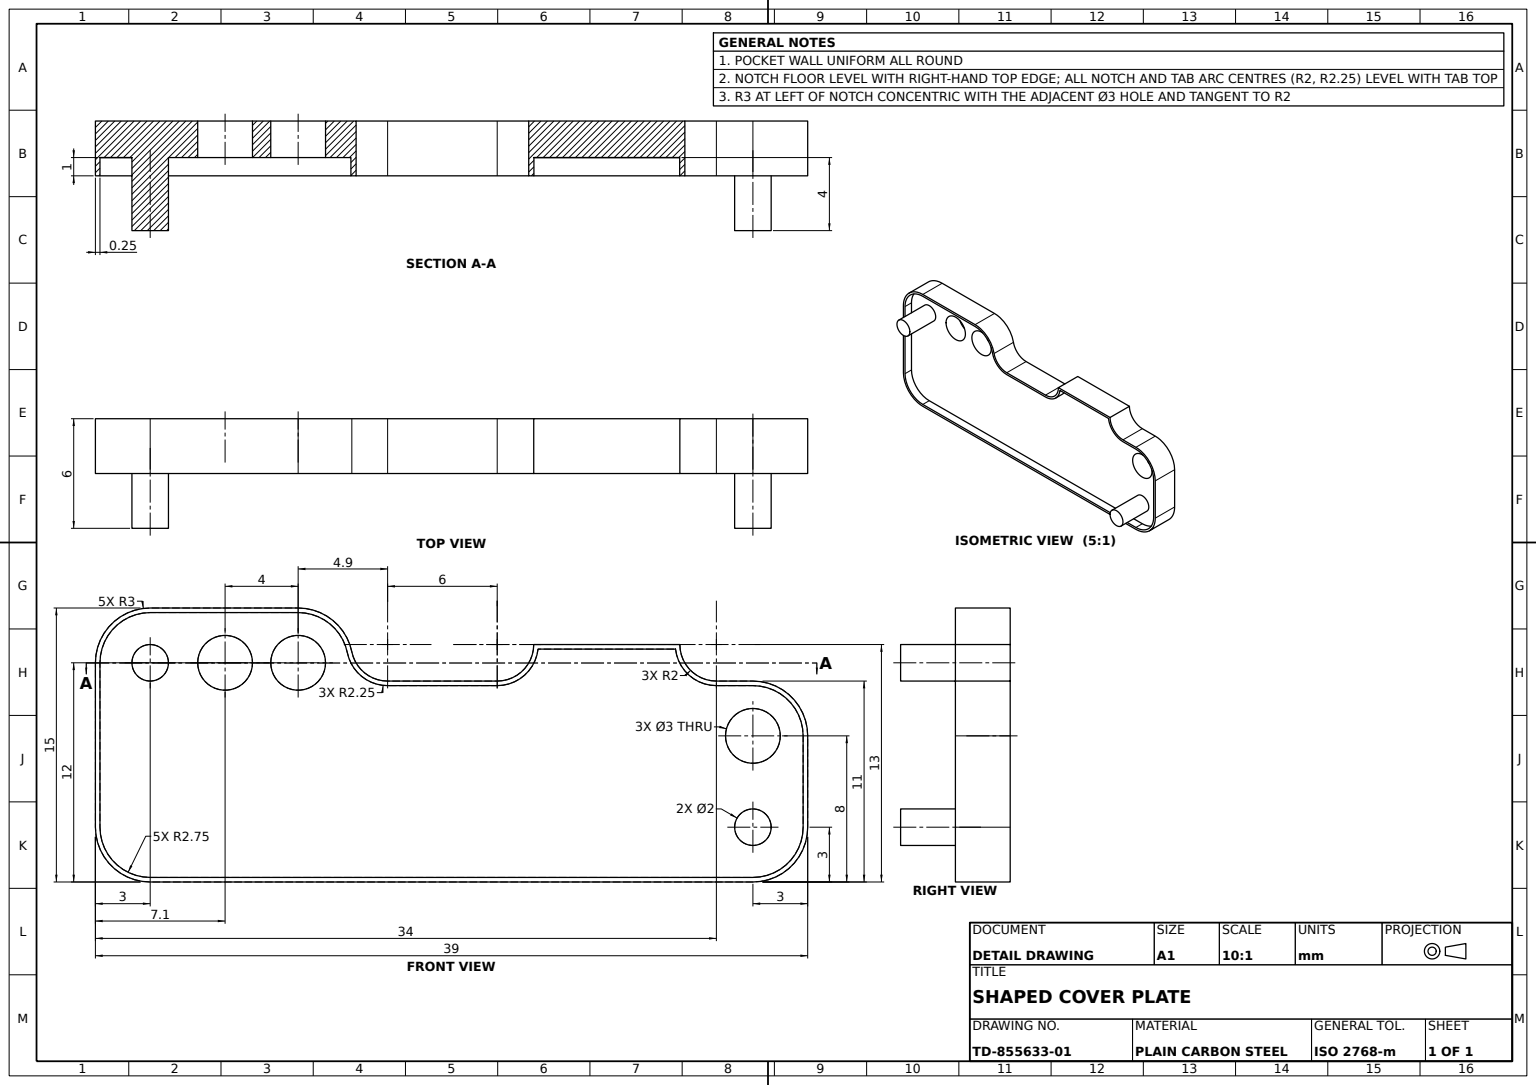
from build123d import *

# Parameters (mm, degrees)
BASE_PLATE_DEPTH         = 2
PERIMETER_RIM_DEPTH      = 1
PIN_1_SKETCH_R           = 1
PIN_1_2_DEPTH            = 4
PIN_2_SKETCH_R           = 1
PIN_2_2_DEPTH            = 4
THROUGH_HOLES_SKETCH_R   = 1.5
THROUGH_HOLES_3X_3_DEPTH = 4


with BuildPart() as part:
    # Base Plate Sketch → Base Plate (new body)
    with BuildSketch(Plane.XY):
        with BuildLine():
            Line((0, 3), (0, 12))
            ThreePointArc((0, 12), (0.878679656, 14.121320344), (3, 15))
            Line((3, 15), (11.101020514, 15))
            ThreePointArc((11.101020514, 15), (12.998387111, 14.323790008), (14.040408206, 12.6))
            ThreePointArc((14.040408206, 12.6), (14.735088936, 11.450806662), (16, 11))
            Line((16, 11), (22, 11))
            ThreePointArc((22, 11), (23.414213562, 11.585786438), (24, 13))
            Line((24, 13), (32, 13))
            ThreePointArc((32, 13), (32.585786438, 11.585786438), (34, 11))
            Line((34, 11), (36, 11))
            ThreePointArc((36, 11), (38.121320344, 10.121320344), (39, 8))
            Line((39, 8), (39, 3))
            ThreePointArc((39, 3), (38.121320344, 0.878679656), (36, 0))
            Line((36, 0), (3, 0))
            ThreePointArc((3, 0), (0.878679656, 0.878679656), (0, 3))
        make_face()
    extrude(amount=BASE_PLATE_DEPTH)

    # Perimeter Rim Sketch → Perimeter Rim (add)
    with BuildSketch(Plane.XY.offset(2)):
        with BuildLine():
            Line((32, 13), (24, 13))
            ThreePointArc((24, 13), (23.414213562, 11.585786438), (22, 11))
            Line((22, 11), (16, 11))
            ThreePointArc((16, 11), (14.735088936, 11.450806662), (14.040408206, 12.6))
            ThreePointArc((14.040408206, 12.6), (12.998387111, 14.323790008), (11.101020514, 15))
            Line((11.101020514, 15), (3, 15))
            ThreePointArc((3, 15), (0.878679656, 14.121320344), (0, 12))
            Line((0, 12), (0, 3))
            ThreePointArc((0, 3), (0.878679656, 0.878679656), (3, 0))
            Line((3, 0), (36, 0))
            ThreePointArc((36, 0), (38.121320344, 0.878679656), (39, 3))
            Line((39, 3), (39, 8))
            ThreePointArc((39, 8), (38.121320344, 10.121320344), (36, 11))
            Line((36, 11), (34, 11))
            ThreePointArc((34, 11), (32.585786438, 11.585786438), (32, 13))
        make_face()
        with BuildLine():
            Line((31.763932023, 12.75), (24.236067977, 12.75))
            ThreePointArc((24.236067977, 12.75), (23.5, 11.322949017), (22, 10.75))
            Line((22, 10.75), (16, 10.75))
            ThreePointArc((16, 10.75), (14.576975053, 11.257157494), (13.795459231, 12.55))
            ThreePointArc((13.795459231, 12.55), (12.840273228, 14.13014084), (11.101020514, 14.75))
            Line((11.101020514, 14.75), (3, 14.75))
            ThreePointArc((3, 14.75), (1.055456352, 13.944543648), (0.25, 12))
            Line((0.25, 12), (0.25, 3))
            ThreePointArc((0.25, 3), (1.055456352, 1.055456352), (3, 0.25))
            Line((3, 0.25), (36, 0.25))
            ThreePointArc((36, 0.25), (37.944543648, 1.055456352), (38.75, 3))
            Line((38.75, 3), (38.75, 8))
            ThreePointArc((38.75, 8), (37.944543648, 9.944543648), (36, 10.75))
            Line((36, 10.75), (34, 10.75))
            ThreePointArc((34, 10.75), (32.5, 11.322949017), (31.763932023, 12.75))
        make_face(mode=Mode.SUBTRACT)
    extrude(amount=PERIMETER_RIM_DEPTH)

    # Pin 1 Sketch → Pin 1 Ø2 (add)
    with BuildSketch(Plane.XY.offset(2)):
        with Locations((36, 3)):
            Circle(PIN_1_SKETCH_R)
    extrude(amount=PIN_1_2_DEPTH)

    # Pin 2 Sketch → Pin 2 Ø2 (add)
    with BuildSketch(Plane.XY.offset(2)):
        with Locations((3, 12)):
            Circle(PIN_2_SKETCH_R)
    extrude(amount=PIN_2_2_DEPTH)

    # Through Holes Sketch → Through Holes 3xØ3 (cut)
    with BuildSketch(Plane.XY.offset(2)):
        with Locations((36, 8)):
            Circle(THROUGH_HOLES_SKETCH_R)
        with Locations((11.101020514, 12)):
            Circle(THROUGH_HOLES_SKETCH_R)
        with Locations((7.101020514, 12)):
            Circle(THROUGH_HOLES_SKETCH_R)
    extrude(amount=-THROUGH_HOLES_3X_3_DEPTH, mode=Mode.SUBTRACT)


solid = part.part
